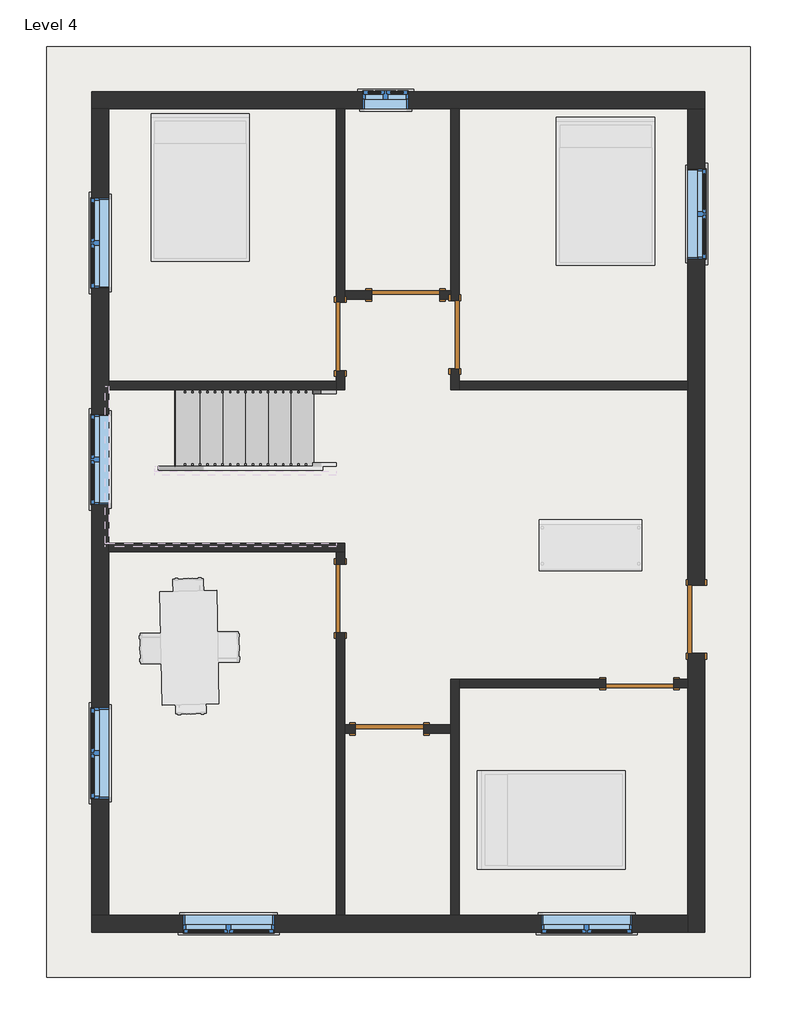
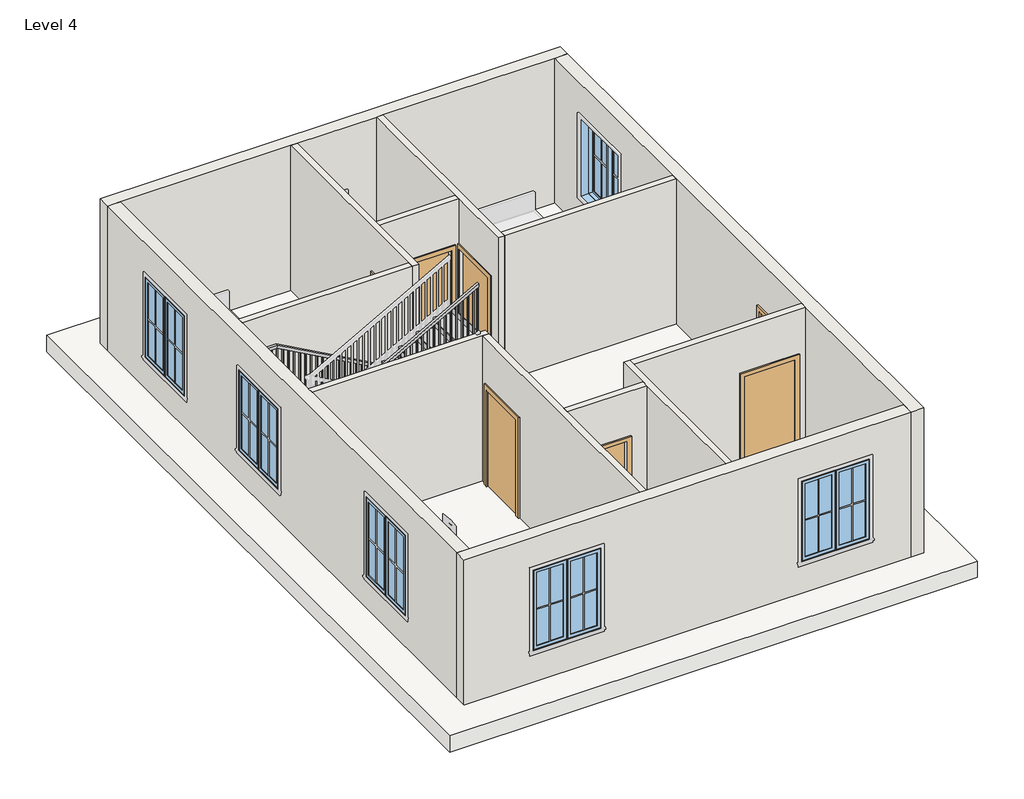
# One storey, part 1 of 2: 14 walls, 7 doors, 7 windows, 1 railing, 1 roof, 1 stair flight.
"""IFC4 building model written with IfcOpenShell, lengths in millimetres."""

from ifc_helpers import new_model, si_unit, frame, origin, place, context, project, spatial, polyline, outline, extrude, faceted_brep, transform, mapped, element, save
from components import door_e5f9f3c4, door_305aa2a5, door_a90ba1ad, stair_flight_3672e095, window_c417fced, window_8377141f

model = new_model("IFC4")

# Units and contexts
model_context = context("Model", 3, world=origin())
ifc_project = project(units=[si_unit("LENGTHUNIT", "METRE", prefix="MILLI")], contexts=[model_context])

# Site, building, storey
site = spatial("IfcSite", under=ifc_project)
building = spatial("IfcBuilding", under=site)
storey = spatial("IfcBuildingStorey", under=building, Name="Level 4", Elevation=9144.0)

# Doors
placement = place(None, origin())
door_shape = door_e5f9f3c4(model_context)
element("IfcDoor", 1, ObjectType="Single-Flush : 36\" x 84\"", at=placement, inside=storey, context=model_context, shape_type="MappedRepresentation", body=[
    mapped(door_shape, transform((5226.05, 11245.85, 9144.0), x_axis=(1.0, 0.0, 0.0), y_axis=(0.0, 1.0, 0.0), z_axis=(0.0, 0.0, 1.0))),
])
element("IfcDoor", 2, ObjectType="Single-Flush : 36\" x 84\"", at=placement, inside=storey, context=model_context, shape_type="MappedRepresentation", body=[
    mapped(door_shape, transform((5886.45, 10712.45, 9144.0), x_axis=(0.0, -1.0, 0.0), y_axis=(1.0, 0.0, 0.0), z_axis=(0.0, 0.0, 1.0))),
])
door_2_shape = door_305aa2a5(model_context)
element("IfcDoor", 3, ObjectType="Single-Flush : 36\" x 84\"", at=placement, inside=storey, context=model_context, shape_type="MappedRepresentation", body=[
    mapped(door_2_shape, transform((4349.75, 10687.05, 9144.0), x_axis=(0.0, -1.0, 0.0), y_axis=(1.0, 0.0, 0.0), z_axis=(0.0, 0.0, 1.0))),
])
element("IfcDoor", 4, ObjectType="Single-Flush : 36\" x 84\"", at=placement, inside=storey, context=model_context, shape_type="MappedRepresentation", body=[
    mapped(door_2_shape, transform((8369.3, 6026.15, 9144.0), x_axis=(1.0, 0.0, 0.0), y_axis=(0.0, 1.0, 0.0), z_axis=(0.0, 0.0, 1.0))),
])
element("IfcDoor", 5, ObjectType="Single-Flush : 36\" x 84\"", at=placement, inside=storey, context=model_context, shape_type="MappedRepresentation", body=[
    mapped(door_2_shape, transform((5010.15, 5416.55, 9144.0), x_axis=(-1.0, 0.0, 0.0), y_axis=(0.0, -1.0, 0.0), z_axis=(0.0, 0.0, 1.0))),
])
element("IfcDoor", 6, ObjectType="Single-Flush : 36\" x 84\"", at=placement, inside=storey, context=model_context, shape_type="MappedRepresentation", body=[
    mapped(door_2_shape, transform((4349.75, 7169.15, 9144.0), x_axis=(0.0, -1.0, 0.0), y_axis=(1.0, 0.0, 0.0), z_axis=(0.0, 0.0, 1.0))),
])
door_3_shape = door_a90ba1ad(model_context)
element("IfcDoor", 7, ObjectType="Single-Flush : 36\" x 84\"", at=placement, inside=storey, context=model_context, shape_type="MappedRepresentation", body=[
    mapped(door_3_shape, transform((9131.3, 6889.75, 9144.0), x_axis=(0.0, -1.0, 0.0), y_axis=(1.0, 0.0, 0.0), z_axis=(0.0, 0.0, 1.0))),
])

# Railing
element("IfcRailing", 8, ObjectType="Handrail - Rectangular", at=placement, inside=storey, context=model_context, shape_type="SolidModel", body=[
    faceted_brep([(4295.1355783, 9918.7, 10227.7333333), (4295.1355783, 9918.7, 10169.620221), (4295.1355783, 9969.5, 10169.620221), (4295.1355783, 9969.5, 10227.7333333), (1856.7355783, 9918.7, 11582.4), (1843.5719761, 9918.7, 11531.6), (1843.5719761, 9969.5, 11531.6), (1856.7355783, 9969.5, 11582.4), (1295.4, 9918.7, 11582.4), (1295.4, 9918.7, 11531.6), (1244.6, 9969.5, 11531.6), (1244.6, 9969.5, 11582.4), (1295.4, 7962.9, 11582.4), (1295.4, 7962.9, 11531.6), (1244.6, 7912.1, 11531.6), (1244.6, 7912.1, 11582.4), (1551.9355783, 7962.9, 11582.4), (1565.0991806, 7962.9, 11531.6), (1565.0991806, 7912.1, 11531.6), (1551.9355783, 7912.1, 11582.4), (4295.1355783, 7962.9, 13106.4), (4295.1355783, 7912.1, 13106.4), (4295.1355783, 7912.1, 13048.2868876), (4295.1355783, 7962.9, 13048.2868876)], [[[0, 1, 2, 3]], [[1, 0, 4, 5]], [[2, 1, 5, 6]], [[3, 2, 6, 7]], [[0, 3, 7, 4]], [[5, 4, 8, 9]], [[6, 5, 9, 10]], [[7, 6, 10, 11]], [[4, 7, 11, 8]], [[9, 8, 12, 13]], [[10, 9, 13, 14]], [[11, 10, 14, 15]], [[8, 11, 15, 12]], [[13, 12, 16, 17]], [[14, 13, 17, 18]], [[15, 14, 18, 19]], [[12, 15, 19, 16]], [[20, 21, 22, 23]], [[17, 16, 20, 23]], [[18, 17, 23, 22]], [[19, 18, 22, 21]], [[16, 19, 21, 20]]]),
    extrude(outline(polyline([(13009.8365664, 4225.925), (12999.253233, 4206.875), (12022.6666667, 4206.875), (12022.6666667, 4225.925), (13009.8365664, 4225.925)])), frame((0.0, 7927.975, 0.0), z_axis=(0.0, 1.0, 0.0), x_axis=(0.0, 0.0, 1.0)), (0.0, 0.0, 1.0), 19.05),
    extrude(outline(polyline([(12953.3921219, 4124.325), (12942.8087886, 4105.275), (12022.6666667, 4105.275), (12022.6666667, 4124.325), (12953.3921219, 4124.325)])), frame((0.0, 7927.975, 0.0), z_axis=(0.0, 1.0, 0.0), x_axis=(0.0, 0.0, 1.0)), (0.0, 0.0, 1.0), 19.05),
    extrude(outline(polyline([(12896.9476775, 4022.725), (12886.3643441, 4003.675), (12022.6666667, 4003.675), (12022.6666667, 4022.725), (12896.9476775, 4022.725)])), frame((0.0, 7927.975, 0.0), z_axis=(0.0, 1.0, 0.0), x_axis=(0.0, 0.0, 1.0)), (0.0, 0.0, 1.0), 19.05),
    extrude(outline(polyline([(12840.503233, 3921.125), (12829.9198997, 3902.075), (11853.3333333, 3902.075), (11853.3333333, 3921.125), (12840.503233, 3921.125)])), frame((0.0, 7927.975, 0.0), z_axis=(0.0, 1.0, 0.0), x_axis=(0.0, 0.0, 1.0)), (0.0, 0.0, 1.0), 19.05),
    extrude(outline(polyline([(12784.0587886, 3819.525), (12773.4754552, 3800.475), (11853.3333333, 3800.475), (11853.3333333, 3819.525), (12784.0587886, 3819.525)])), frame((0.0, 7927.975, 0.0), z_axis=(0.0, 1.0, 0.0), x_axis=(0.0, 0.0, 1.0)), (0.0, 0.0, 1.0), 19.05),
    extrude(outline(polyline([(12727.6143441, 3717.925), (12717.0310108, 3698.875), (11853.3333333, 3698.875), (11853.3333333, 3717.925), (12727.6143441, 3717.925)])), frame((0.0, 7927.975, 0.0), z_axis=(0.0, 1.0, 0.0), x_axis=(0.0, 0.0, 1.0)), (0.0, 0.0, 1.0), 19.05),
    extrude(outline(polyline([(12671.1698997, 3616.325), (12660.5865664, 3597.275), (11684.0, 3597.275), (11684.0, 3616.325), (12671.1698997, 3616.325)])), frame((0.0, 7927.975, 0.0), z_axis=(0.0, 1.0, 0.0), x_axis=(0.0, 0.0, 1.0)), (0.0, 0.0, 1.0), 19.05),
    extrude(outline(polyline([(12614.7254552, 3514.725), (12604.1421219, 3495.675), (11684.0, 3495.675), (11684.0, 3514.725), (12614.7254552, 3514.725)])), frame((0.0, 7927.975, 0.0), z_axis=(0.0, 1.0, 0.0), x_axis=(0.0, 0.0, 1.0)), (0.0, 0.0, 1.0), 19.05),
    extrude(outline(polyline([(12558.2810108, 3413.125), (12547.6976775, 3394.075), (11684.0, 3394.075), (11684.0, 3413.125), (12558.2810108, 3413.125)])), frame((0.0, 7927.975, 0.0), z_axis=(0.0, 1.0, 0.0), x_axis=(0.0, 0.0, 1.0)), (0.0, 0.0, 1.0), 19.05),
    extrude(outline(polyline([(12501.8365664, 3311.525), (12491.253233, 3292.475), (11514.6666667, 3292.475), (11514.6666667, 3311.525), (12501.8365664, 3311.525)])), frame((0.0, 7927.975, 0.0), z_axis=(0.0, 1.0, 0.0), x_axis=(0.0, 0.0, 1.0)), (0.0, 0.0, 1.0), 19.05),
    extrude(outline(polyline([(12445.3921219, 3209.925), (12434.8087886, 3190.875), (11514.6666667, 3190.875), (11514.6666667, 3209.925), (12445.3921219, 3209.925)])), frame((0.0, 7927.975, 0.0), z_axis=(0.0, 1.0, 0.0), x_axis=(0.0, 0.0, 1.0)), (0.0, 0.0, 1.0), 19.05),
    extrude(outline(polyline([(12388.9476775, 3108.325), (12378.3643441, 3089.275), (11514.6666667, 3089.275), (11514.6666667, 3108.325), (12388.9476775, 3108.325)])), frame((0.0, 7927.975, 0.0), z_axis=(0.0, 1.0, 0.0), x_axis=(0.0, 0.0, 1.0)), (0.0, 0.0, 1.0), 19.05),
    extrude(outline(polyline([(12332.503233, 3006.725), (12321.9198997, 2987.675), (11345.3333333, 2987.675), (11345.3333333, 3006.725), (12332.503233, 3006.725)])), frame((0.0, 7927.975, 0.0), z_axis=(0.0, 1.0, 0.0), x_axis=(0.0, 0.0, 1.0)), (0.0, 0.0, 1.0), 19.05),
    extrude(outline(polyline([(12276.0587886, 2905.125), (12265.4754552, 2886.075), (11345.3333333, 2886.075), (11345.3333333, 2905.125), (12276.0587886, 2905.125)])), frame((0.0, 7927.975, 0.0), z_axis=(0.0, 1.0, 0.0), x_axis=(0.0, 0.0, 1.0)), (0.0, 0.0, 1.0), 19.05),
    extrude(outline(polyline([(12219.6143441, 2803.525), (12209.0310108, 2784.475), (11345.3333333, 2784.475), (11345.3333333, 2803.525), (12219.6143441, 2803.525)])), frame((0.0, 7927.975, 0.0), z_axis=(0.0, 1.0, 0.0), x_axis=(0.0, 0.0, 1.0)), (0.0, 0.0, 1.0), 19.05),
    extrude(outline(polyline([(12163.1698997, 2701.925), (12152.5865664, 2682.875), (11176.0, 2682.875), (11176.0, 2701.925), (12163.1698997, 2701.925)])), frame((0.0, 7927.975, 0.0), z_axis=(0.0, 1.0, 0.0), x_axis=(0.0, 0.0, 1.0)), (0.0, 0.0, 1.0), 19.05),
    extrude(outline(polyline([(12106.7254552, 2600.325), (12096.1421219, 2581.275), (11176.0, 2581.275), (11176.0, 2600.325), (12106.7254552, 2600.325)])), frame((0.0, 7927.975, 0.0), z_axis=(0.0, 1.0, 0.0), x_axis=(0.0, 0.0, 1.0)), (0.0, 0.0, 1.0), 19.05),
    extrude(outline(polyline([(12050.2810108, 2498.725), (12039.6976775, 2479.675), (11176.0, 2479.675), (11176.0, 2498.725), (12050.2810108, 2498.725)])), frame((0.0, 7927.975, 0.0), z_axis=(0.0, 1.0, 0.0), x_axis=(0.0, 0.0, 1.0)), (0.0, 0.0, 1.0), 19.05),
    extrude(outline(polyline([(11993.8365664, 2397.125), (11983.253233, 2378.075), (11006.6666667, 2378.075), (11006.6666667, 2397.125), (11993.8365664, 2397.125)])), frame((0.0, 7927.975, 0.0), z_axis=(0.0, 1.0, 0.0), x_axis=(0.0, 0.0, 1.0)), (0.0, 0.0, 1.0), 19.05),
    extrude(outline(polyline([(11937.3921219, 2295.525), (11926.8087886, 2276.475), (11006.6666667, 2276.475), (11006.6666667, 2295.525), (11937.3921219, 2295.525)])), frame((0.0, 7927.975, 0.0), z_axis=(0.0, 1.0, 0.0), x_axis=(0.0, 0.0, 1.0)), (0.0, 0.0, 1.0), 19.05),
    extrude(outline(polyline([(11880.9476775, 2193.925), (11870.3643441, 2174.875), (11006.6666667, 2174.875), (11006.6666667, 2193.925), (11880.9476775, 2193.925)])), frame((0.0, 7927.975, 0.0), z_axis=(0.0, 1.0, 0.0), x_axis=(0.0, 0.0, 1.0)), (0.0, 0.0, 1.0), 19.05),
    extrude(outline(polyline([(11824.503233, 2092.325), (11813.9198997, 2073.275), (10837.3333333, 2073.275), (10837.3333333, 2092.325), (11824.503233, 2092.325)])), frame((0.0, 7927.975, 0.0), z_axis=(0.0, 1.0, 0.0), x_axis=(0.0, 0.0, 1.0)), (0.0, 0.0, 1.0), 19.05),
    extrude(outline(polyline([(11768.0587886, 1990.725), (11757.4754552, 1971.675), (10837.3333333, 1971.675), (10837.3333333, 1990.725), (11768.0587886, 1990.725)])), frame((0.0, 7927.975, 0.0), z_axis=(0.0, 1.0, 0.0), x_axis=(0.0, 0.0, 1.0)), (0.0, 0.0, 1.0), 19.05),
    extrude(outline(polyline([(11711.6143441, 1889.125), (11701.0310108, 1870.075), (10837.3333333, 1870.075), (10837.3333333, 1889.125), (11711.6143441, 1889.125)])), frame((0.0, 7927.975, 0.0), z_axis=(0.0, 1.0, 0.0), x_axis=(0.0, 0.0, 1.0)), (0.0, 0.0, 1.0), 19.05),
    extrude(outline(polyline([(11655.1698997, 1787.525), (11644.5865664, 1768.475), (10668.0, 1768.475), (10668.0, 1787.525), (11655.1698997, 1787.525)])), frame((0.0, 7927.975, 0.0), z_axis=(0.0, 1.0, 0.0), x_axis=(0.0, 0.0, 1.0)), (0.0, 0.0, 1.0), 19.05),
    extrude(outline(polyline([(11598.7254552, 1685.925), (11588.1421219, 1666.875), (10668.0, 1666.875), (10668.0, 1685.925), (11598.7254552, 1685.925)])), frame((0.0, 7927.975, 0.0), z_axis=(0.0, 1.0, 0.0), x_axis=(0.0, 0.0, 1.0)), (0.0, 0.0, 1.0), 19.05),
    extrude(outline(polyline([(11542.2810108, 1584.325), (11531.6976775, 1565.275), (10668.0, 1565.275), (10668.0, 1584.325), (11542.2810108, 1584.325)])), frame((0.0, 7927.975, 0.0), z_axis=(0.0, 1.0, 0.0), x_axis=(0.0, 0.0, 1.0)), (0.0, 0.0, 1.0), 19.05),
    extrude(outline(polyline([(1463.675, 7927.975), (1463.675, 7947.025), (1482.725, 7947.025), (1482.725, 7927.975), (1463.675, 7927.975)])), frame((0.0, 0.0, 10668.0), z_axis=(0.0, 0.0, 1.0), x_axis=(1.0, 0.0, 0.0)), (0.0, 0.0, 1.0), 863.6),
    extrude(outline(polyline([(1362.075, 7927.975), (1362.075, 7947.025), (1381.125, 7947.025), (1381.125, 7927.975), (1362.075, 7927.975)])), frame((0.0, 0.0, 10668.0), z_axis=(0.0, 0.0, 1.0), x_axis=(1.0, 0.0, 0.0)), (0.0, 0.0, 1.0), 863.6),
    extrude(outline(polyline([(1260.475, 8023.225), (1279.525, 8023.225), (1279.525, 8004.175), (1260.475, 8004.175), (1260.475, 8023.225)])), frame((0.0, 0.0, 10668.0), z_axis=(0.0, 0.0, 1.0), x_axis=(1.0, 0.0, 0.0)), (0.0, 0.0, 1.0), 863.6),
    extrude(outline(polyline([(1260.475, 8124.825), (1279.525, 8124.825), (1279.525, 8105.775), (1260.475, 8105.775), (1260.475, 8124.825)])), frame((0.0, 0.0, 10668.0), z_axis=(0.0, 0.0, 1.0), x_axis=(1.0, 0.0, 0.0)), (0.0, 0.0, 1.0), 863.6),
    extrude(outline(polyline([(1260.475, 8226.425), (1279.525, 8226.425), (1279.525, 8207.375), (1260.475, 8207.375), (1260.475, 8226.425)])), frame((0.0, 0.0, 10668.0), z_axis=(0.0, 0.0, 1.0), x_axis=(1.0, 0.0, 0.0)), (0.0, 0.0, 1.0), 863.6),
    extrude(outline(polyline([(1260.475, 8328.025), (1279.525, 8328.025), (1279.525, 8308.975), (1260.475, 8308.975), (1260.475, 8328.025)])), frame((0.0, 0.0, 10668.0), z_axis=(0.0, 0.0, 1.0), x_axis=(1.0, 0.0, 0.0)), (0.0, 0.0, 1.0), 863.6),
    extrude(outline(polyline([(1260.475, 8429.625), (1279.525, 8429.625), (1279.525, 8410.575), (1260.475, 8410.575), (1260.475, 8429.625)])), frame((0.0, 0.0, 10668.0), z_axis=(0.0, 0.0, 1.0), x_axis=(1.0, 0.0, 0.0)), (0.0, 0.0, 1.0), 863.6),
    extrude(outline(polyline([(1260.475, 8531.225), (1279.525, 8531.225), (1279.525, 8512.175), (1260.475, 8512.175), (1260.475, 8531.225)])), frame((0.0, 0.0, 10668.0), z_axis=(0.0, 0.0, 1.0), x_axis=(1.0, 0.0, 0.0)), (0.0, 0.0, 1.0), 863.6),
    extrude(outline(polyline([(1260.475, 8632.825), (1279.525, 8632.825), (1279.525, 8613.775), (1260.475, 8613.775), (1260.475, 8632.825)])), frame((0.0, 0.0, 10668.0), z_axis=(0.0, 0.0, 1.0), x_axis=(1.0, 0.0, 0.0)), (0.0, 0.0, 1.0), 863.6),
    extrude(outline(polyline([(1260.475, 8734.425), (1279.525, 8734.425), (1279.525, 8715.375), (1260.475, 8715.375), (1260.475, 8734.425)])), frame((0.0, 0.0, 10668.0), z_axis=(0.0, 0.0, 1.0), x_axis=(1.0, 0.0, 0.0)), (0.0, 0.0, 1.0), 863.6),
    extrude(outline(polyline([(1260.475, 8836.025), (1279.525, 8836.025), (1279.525, 8816.975), (1260.475, 8816.975), (1260.475, 8836.025)])), frame((0.0, 0.0, 10668.0), z_axis=(0.0, 0.0, 1.0), x_axis=(1.0, 0.0, 0.0)), (0.0, 0.0, 1.0), 863.6),
    extrude(outline(polyline([(1260.475, 8937.625), (1279.525, 8937.625), (1279.525, 8918.575), (1260.475, 8918.575), (1260.475, 8937.625)])), frame((0.0, 0.0, 10668.0), z_axis=(0.0, 0.0, 1.0), x_axis=(1.0, 0.0, 0.0)), (0.0, 0.0, 1.0), 863.6),
    extrude(outline(polyline([(1260.475, 9039.225), (1279.525, 9039.225), (1279.525, 9020.175), (1260.475, 9020.175), (1260.475, 9039.225)])), frame((0.0, 0.0, 10668.0), z_axis=(0.0, 0.0, 1.0), x_axis=(1.0, 0.0, 0.0)), (0.0, 0.0, 1.0), 863.6),
    extrude(outline(polyline([(1260.475, 9140.825), (1279.525, 9140.825), (1279.525, 9121.775), (1260.475, 9121.775), (1260.475, 9140.825)])), frame((0.0, 0.0, 10668.0), z_axis=(0.0, 0.0, 1.0), x_axis=(1.0, 0.0, 0.0)), (0.0, 0.0, 1.0), 863.6),
    extrude(outline(polyline([(1260.475, 9242.425), (1279.525, 9242.425), (1279.525, 9223.375), (1260.475, 9223.375), (1260.475, 9242.425)])), frame((0.0, 0.0, 10668.0), z_axis=(0.0, 0.0, 1.0), x_axis=(1.0, 0.0, 0.0)), (0.0, 0.0, 1.0), 863.6),
    extrude(outline(polyline([(1260.475, 9344.025), (1279.525, 9344.025), (1279.525, 9324.975), (1260.475, 9324.975), (1260.475, 9344.025)])), frame((0.0, 0.0, 10668.0), z_axis=(0.0, 0.0, 1.0), x_axis=(1.0, 0.0, 0.0)), (0.0, 0.0, 1.0), 863.6),
    extrude(outline(polyline([(1260.475, 9445.625), (1279.525, 9445.625), (1279.525, 9426.575), (1260.475, 9426.575), (1260.475, 9445.625)])), frame((0.0, 0.0, 10668.0), z_axis=(0.0, 0.0, 1.0), x_axis=(1.0, 0.0, 0.0)), (0.0, 0.0, 1.0), 863.6),
    extrude(outline(polyline([(1260.475, 9547.225), (1279.525, 9547.225), (1279.525, 9528.175), (1260.475, 9528.175), (1260.475, 9547.225)])), frame((0.0, 0.0, 10668.0), z_axis=(0.0, 0.0, 1.0), x_axis=(1.0, 0.0, 0.0)), (0.0, 0.0, 1.0), 863.6),
    extrude(outline(polyline([(1260.475, 9648.825), (1279.525, 9648.825), (1279.525, 9629.775), (1260.475, 9629.775), (1260.475, 9648.825)])), frame((0.0, 0.0, 10668.0), z_axis=(0.0, 0.0, 1.0), x_axis=(1.0, 0.0, 0.0)), (0.0, 0.0, 1.0), 863.6),
    extrude(outline(polyline([(1260.475, 9750.425), (1279.525, 9750.425), (1279.525, 9731.375), (1260.475, 9731.375), (1260.475, 9750.425)])), frame((0.0, 0.0, 10668.0), z_axis=(0.0, 0.0, 1.0), x_axis=(1.0, 0.0, 0.0)), (0.0, 0.0, 1.0), 863.6),
    extrude(outline(polyline([(1260.475, 9852.025), (1279.525, 9852.025), (1279.525, 9832.975), (1260.475, 9832.975), (1260.475, 9852.025)])), frame((0.0, 0.0, 10668.0), z_axis=(0.0, 0.0, 1.0), x_axis=(1.0, 0.0, 0.0)), (0.0, 0.0, 1.0), 863.6),
    extrude(outline(polyline([(1358.2605783, 9953.625), (1358.2605783, 9934.575), (1339.2105783, 9934.575), (1339.2105783, 9953.625), (1358.2605783, 9953.625)])), frame((0.0, 0.0, 10668.0), z_axis=(0.0, 0.0, 1.0), x_axis=(1.0, 0.0, 0.0)), (0.0, 0.0, 1.0), 863.6),
    extrude(outline(polyline([(1459.8605783, 9953.625), (1459.8605783, 9934.575), (1440.8105783, 9934.575), (1440.8105783, 9953.625), (1459.8605783, 9953.625)])), frame((0.0, 0.0, 10668.0), z_axis=(0.0, 0.0, 1.0), x_axis=(1.0, 0.0, 0.0)), (0.0, 0.0, 1.0), 863.6),
    extrude(outline(polyline([(1561.4605783, 9953.625), (1561.4605783, 9934.575), (1542.4105783, 9934.575), (1542.4105783, 9953.625), (1561.4605783, 9953.625)])), frame((0.0, 0.0, 10668.0), z_axis=(0.0, 0.0, 1.0), x_axis=(1.0, 0.0, 0.0)), (0.0, 0.0, 1.0), 863.6),
    extrude(outline(polyline([(1663.0605783, 9953.625), (1663.0605783, 9934.575), (1644.0105783, 9934.575), (1644.0105783, 9953.625), (1663.0605783, 9953.625)])), frame((0.0, 0.0, 10668.0), z_axis=(0.0, 0.0, 1.0), x_axis=(1.0, 0.0, 0.0)), (0.0, 0.0, 1.0), 863.6),
    extrude(outline(polyline([(1764.6605783, 9953.625), (1764.6605783, 9934.575), (1745.6105783, 9934.575), (1745.6105783, 9953.625), (1764.6605783, 9953.625)])), frame((0.0, 0.0, 10668.0), z_axis=(0.0, 0.0, 1.0), x_axis=(1.0, 0.0, 0.0)), (0.0, 0.0, 1.0), 863.6),
    extrude(outline(polyline([(11518.995221, 1866.2605783), (11529.5785543, 1847.2105783), (10668.0, 1847.2105783), (10668.0, 1866.2605783), (11518.995221, 1866.2605783)])), frame((0.0, 9934.575, 0.0), z_axis=(0.0, 1.0, 0.0), x_axis=(0.0, 0.0, 1.0)), (0.0, 0.0, 1.0), 19.05),
    extrude(outline(polyline([(11462.5507765, 1967.8605783), (11473.1341099, 1948.8105783), (10498.6666667, 1948.8105783), (10498.6666667, 1967.8605783), (11462.5507765, 1967.8605783)])), frame((0.0, 9934.575, 0.0), z_axis=(0.0, 1.0, 0.0), x_axis=(0.0, 0.0, 1.0)), (0.0, 0.0, 1.0), 19.05),
    extrude(outline(polyline([(11406.1063321, 2069.4605783), (11416.6896654, 2050.4105783), (10498.6666667, 2050.4105783), (10498.6666667, 2069.4605783), (11406.1063321, 2069.4605783)])), frame((0.0, 9934.575, 0.0), z_axis=(0.0, 1.0, 0.0), x_axis=(0.0, 0.0, 1.0)), (0.0, 0.0, 1.0), 19.05),
    extrude(outline(polyline([(11349.6618876, 2171.0605783), (11360.245221, 2152.0105783), (10498.6666667, 2152.0105783), (10498.6666667, 2171.0605783), (11349.6618876, 2171.0605783)])), frame((0.0, 9934.575, 0.0), z_axis=(0.0, 1.0, 0.0), x_axis=(0.0, 0.0, 1.0)), (0.0, 0.0, 1.0), 19.05),
    extrude(outline(polyline([(11293.2174432, 2272.6605783), (11303.8007765, 2253.6105783), (10329.3333333, 2253.6105783), (10329.3333333, 2272.6605783), (11293.2174432, 2272.6605783)])), frame((0.0, 9934.575, 0.0), z_axis=(0.0, 1.0, 0.0), x_axis=(0.0, 0.0, 1.0)), (0.0, 0.0, 1.0), 19.05),
    extrude(outline(polyline([(11236.7729988, 2374.2605783), (11247.3563321, 2355.2105783), (10329.3333333, 2355.2105783), (10329.3333333, 2374.2605783), (11236.7729988, 2374.2605783)])), frame((0.0, 9934.575, 0.0), z_axis=(0.0, 1.0, 0.0), x_axis=(0.0, 0.0, 1.0)), (0.0, 0.0, 1.0), 19.05),
    extrude(outline(polyline([(11180.3285543, 2475.8605783), (11190.9118876, 2456.8105783), (10329.3333333, 2456.8105783), (10329.3333333, 2475.8605783), (11180.3285543, 2475.8605783)])), frame((0.0, 9934.575, 0.0), z_axis=(0.0, 1.0, 0.0), x_axis=(0.0, 0.0, 1.0)), (0.0, 0.0, 1.0), 19.05),
    extrude(outline(polyline([(11123.8841099, 2577.4605783), (11134.4674432, 2558.4105783), (10160.0, 2558.4105783), (10160.0, 2577.4605783), (11123.8841099, 2577.4605783)])), frame((0.0, 9934.575, 0.0), z_axis=(0.0, 1.0, 0.0), x_axis=(0.0, 0.0, 1.0)), (0.0, 0.0, 1.0), 19.05),
    extrude(outline(polyline([(11067.4396654, 2679.0605783), (11078.0229988, 2660.0105783), (10160.0, 2660.0105783), (10160.0, 2679.0605783), (11067.4396654, 2679.0605783)])), frame((0.0, 9934.575, 0.0), z_axis=(0.0, 1.0, 0.0), x_axis=(0.0, 0.0, 1.0)), (0.0, 0.0, 1.0), 19.05),
    extrude(outline(polyline([(11010.995221, 2780.6605783), (11021.5785543, 2761.6105783), (10160.0, 2761.6105783), (10160.0, 2780.6605783), (11010.995221, 2780.6605783)])), frame((0.0, 9934.575, 0.0), z_axis=(0.0, 1.0, 0.0), x_axis=(0.0, 0.0, 1.0)), (0.0, 0.0, 1.0), 19.05),
    extrude(outline(polyline([(10954.5507765, 2882.2605783), (10965.1341099, 2863.2105783), (9990.6666667, 2863.2105783), (9990.6666667, 2882.2605783), (10954.5507765, 2882.2605783)])), frame((0.0, 9934.575, 0.0), z_axis=(0.0, 1.0, 0.0), x_axis=(0.0, 0.0, 1.0)), (0.0, 0.0, 1.0), 19.05),
    extrude(outline(polyline([(10898.1063321, 2983.8605783), (10908.6896654, 2964.8105783), (9990.6666667, 2964.8105783), (9990.6666667, 2983.8605783), (10898.1063321, 2983.8605783)])), frame((0.0, 9934.575, 0.0), z_axis=(0.0, 1.0, 0.0), x_axis=(0.0, 0.0, 1.0)), (0.0, 0.0, 1.0), 19.05),
    extrude(outline(polyline([(10841.6618876, 3085.4605783), (10852.245221, 3066.4105783), (9990.6666667, 3066.4105783), (9990.6666667, 3085.4605783), (10841.6618876, 3085.4605783)])), frame((0.0, 9934.575, 0.0), z_axis=(0.0, 1.0, 0.0), x_axis=(0.0, 0.0, 1.0)), (0.0, 0.0, 1.0), 19.05),
    extrude(outline(polyline([(10785.2174432, 3187.0605783), (10795.8007765, 3168.0105783), (9821.3333333, 3168.0105783), (9821.3333333, 3187.0605783), (10785.2174432, 3187.0605783)])), frame((0.0, 9934.575, 0.0), z_axis=(0.0, 1.0, 0.0), x_axis=(0.0, 0.0, 1.0)), (0.0, 0.0, 1.0), 19.05),
    extrude(outline(polyline([(10728.7729988, 3288.6605783), (10739.3563321, 3269.6105783), (9821.3333333, 3269.6105783), (9821.3333333, 3288.6605783), (10728.7729988, 3288.6605783)])), frame((0.0, 9934.575, 0.0), z_axis=(0.0, 1.0, 0.0), x_axis=(0.0, 0.0, 1.0)), (0.0, 0.0, 1.0), 19.05),
    extrude(outline(polyline([(10672.3285543, 3390.2605783), (10682.9118876, 3371.2105783), (9821.3333333, 3371.2105783), (9821.3333333, 3390.2605783), (10672.3285543, 3390.2605783)])), frame((0.0, 9934.575, 0.0), z_axis=(0.0, 1.0, 0.0), x_axis=(0.0, 0.0, 1.0)), (0.0, 0.0, 1.0), 19.05),
    extrude(outline(polyline([(10615.8841099, 3491.8605783), (10626.4674432, 3472.8105783), (9652.0, 3472.8105783), (9652.0, 3491.8605783), (10615.8841099, 3491.8605783)])), frame((0.0, 9934.575, 0.0), z_axis=(0.0, 1.0, 0.0), x_axis=(0.0, 0.0, 1.0)), (0.0, 0.0, 1.0), 19.05),
    extrude(outline(polyline([(10559.4396654, 3593.4605783), (10570.0229988, 3574.4105783), (9652.0, 3574.4105783), (9652.0, 3593.4605783), (10559.4396654, 3593.4605783)])), frame((0.0, 9934.575, 0.0), z_axis=(0.0, 1.0, 0.0), x_axis=(0.0, 0.0, 1.0)), (0.0, 0.0, 1.0), 19.05),
    extrude(outline(polyline([(10502.995221, 3695.0605783), (10513.5785543, 3676.0105783), (9652.0, 3676.0105783), (9652.0, 3695.0605783), (10502.995221, 3695.0605783)])), frame((0.0, 9934.575, 0.0), z_axis=(0.0, 1.0, 0.0), x_axis=(0.0, 0.0, 1.0)), (0.0, 0.0, 1.0), 19.05),
    extrude(outline(polyline([(10446.5507765, 3796.6605783), (10457.1341099, 3777.6105783), (9482.6666667, 3777.6105783), (9482.6666667, 3796.6605783), (10446.5507765, 3796.6605783)])), frame((0.0, 9934.575, 0.0), z_axis=(0.0, 1.0, 0.0), x_axis=(0.0, 0.0, 1.0)), (0.0, 0.0, 1.0), 19.05),
    extrude(outline(polyline([(10390.1063321, 3898.2605783), (10400.6896654, 3879.2105783), (9482.6666667, 3879.2105783), (9482.6666667, 3898.2605783), (10390.1063321, 3898.2605783)])), frame((0.0, 9934.575, 0.0), z_axis=(0.0, 1.0, 0.0), x_axis=(0.0, 0.0, 1.0)), (0.0, 0.0, 1.0), 19.05),
    extrude(outline(polyline([(10333.6618876, 3999.8605783), (10344.245221, 3980.8105783), (9482.6666667, 3980.8105783), (9482.6666667, 3999.8605783), (10333.6618876, 3999.8605783)])), frame((0.0, 9934.575, 0.0), z_axis=(0.0, 1.0, 0.0), x_axis=(0.0, 0.0, 1.0)), (0.0, 0.0, 1.0), 19.05),
    extrude(outline(polyline([(10277.2174432, 4101.4605783), (10287.8007765, 4082.4105783), (9313.3333333, 4082.4105783), (9313.3333333, 4101.4605783), (10277.2174432, 4101.4605783)])), frame((0.0, 9934.575, 0.0), z_axis=(0.0, 1.0, 0.0), x_axis=(0.0, 0.0, 1.0)), (0.0, 0.0, 1.0), 19.05),
    extrude(outline(polyline([(10220.7729988, 4203.0605783), (10231.3563321, 4184.0105783), (9313.3333333, 4184.0105783), (9313.3333333, 4203.0605783), (10220.7729988, 4203.0605783)])), frame((0.0, 9934.575, 0.0), z_axis=(0.0, 1.0, 0.0), x_axis=(0.0, 0.0, 1.0)), (0.0, 0.0, 1.0), 19.05),
    extrude(outline(polyline([(1260.475, 7947.025), (1279.525, 7947.025), (1279.525, 7927.975), (1260.475, 7927.975), (1260.475, 7947.025)])), frame((0.0, 0.0, 10668.0), z_axis=(0.0, 0.0, 1.0), x_axis=(1.0, 0.0, 0.0)), (0.0, 0.0, 1.0), 863.6),
    extrude(outline(polyline([(1279.525, 9953.625), (1279.525, 9934.575), (1260.475, 9934.575), (1260.475, 9953.625), (1279.525, 9953.625)])), frame((0.0, 0.0, 10668.0), z_axis=(0.0, 0.0, 1.0), x_axis=(1.0, 0.0, 0.0)), (0.0, 0.0, 1.0), 863.6),
    extrude(outline(polyline([(13048.2868876, 4295.1355783), (13037.7035543, 4276.0855783), (12022.6666667, 4276.0855783), (12022.6666667, 4295.1355783), (13048.2868876, 4295.1355783)])), frame((0.0, 7927.975, 0.0), z_axis=(0.0, 1.0, 0.0), x_axis=(0.0, 0.0, 1.0)), (0.0, 0.0, 1.0), 19.05),
    extrude(outline(polyline([(10169.620221, 4295.1355783), (10180.2035543, 4276.0855783), (9313.3333333, 4276.0855783), (9313.3333333, 4295.1355783), (10169.620221, 4295.1355783)])), frame((0.0, 9934.575, 0.0), z_axis=(0.0, 1.0, 0.0), x_axis=(0.0, 0.0, 1.0)), (0.0, 0.0, 1.0), 19.05),
])

# Roof
element("IfcRoof", 9, ObjectType="Generic - 12\"", at=placement, inside=storey, context=model_context, shape_type="SweptSolid", body=[
    extrude(outline(polyline([(406.4, 14579.6), (9855.2, 14579.6), (9855.2, 2082.8), (406.4, 2082.8), (406.4, 14579.6)])), frame((0.0, 0.0, 9144.0), z_axis=(0.0, 0.0, 1.0), x_axis=(1.0, 0.0, 0.0)), (0.0, 0.0, 1.0), 304.8),
])

# Stair flight
stair_flight_shape = stair_flight_3672e095(model_context)
element("IfcStairFlight", 10, ObjectType="2\" Tread 1\" Nosing 1/4\" Riser", at=placement, inside=storey, context=model_context, shape_type="MappedRepresentation", body=[
    mapped(stair_flight_shape, transform((0.0, 0.0, 0.0), x_axis=(1.0, 0.0, 0.0), y_axis=(0.0, 1.0, 0.0), z_axis=(0.0, 0.0, 1.0))),
])

# Walls
element("IfcWall", 11, ObjectType="Generic - 5\"", at=placement, inside=storey, context=model_context, shape_type="Brep", body=[
    faceted_brep([(4292.6, 10229.85, 11277.6), (4292.6, 10229.85, 9144.0), (4292.6, 10083.8, 9144.0), (4292.6, 9969.5, 9144.0), (4292.6, 9969.5, 12192.0), (4292.6, 10083.8, 12192.0), (4292.6, 13741.4, 12192.0), (4292.6, 13741.4, 9144.0), (4292.6, 11144.25, 9144.0), (4292.6, 11144.25, 11277.6), (4406.9, 9969.5, 9144.0), (4406.9, 10229.85, 9144.0), (4406.9, 10229.85, 11277.6), (4406.9, 11144.25, 11277.6), (4406.9, 11144.25, 9144.0), (4406.9, 11188.7, 9144.0), (4406.9, 11303.0, 9144.0), (4406.9, 13741.4, 9144.0), (4406.9, 13741.4, 12192.0), (4406.9, 11303.0, 12192.0), (4406.9, 11188.7, 12192.0), (4406.9, 9969.5, 12192.0)], [[[0, 1, 2, 3, 4, 5, 6, 7, 8, 9]], [[10, 11, 12, 13, 14, 15, 16, 17, 18, 19, 20, 21]], [[8, 7, 17, 16, 15, 14]], [[3, 2, 1, 11, 10]], [[6, 5, 4, 21, 20, 19, 18]], [[7, 6, 18, 17]], [[4, 3, 10, 21]], [[12, 11, 1, 0]], [[13, 12, 0, 9]], [[14, 13, 9, 8]]]),
])
element("IfcWall", 12, ObjectType="Generic - 5\"", at=placement, inside=storey, context=model_context, shape_type="SweptSolid", body=[
    extrude(outline(polyline([(1244.6, 10083.8), (4292.6, 10083.8), (4292.6, 9969.5), (1244.6, 9969.5), (1244.6, 10083.8)])), frame((0.0, 0.0, 9144.0), z_axis=(0.0, 0.0, 1.0), x_axis=(1.0, 0.0, 0.0)), (0.0, 0.0, 1.0), 3048.0),
])
element("IfcWall", 13, ObjectType="Generic - 5\"", at=placement, inside=storey, context=model_context, shape_type="SweptSolid", body=[
    extrude(outline(polyline([(11277.6, 5683.25), (9144.0, 5683.25), (9144.0, 5829.3), (12192.0, 5829.3), (12192.0, 4406.9), (9144.0, 4406.9), (9144.0, 4768.85), (11277.6, 4768.85), (11277.6, 5683.25)])), frame((0.0, 11188.7, 0.0), z_axis=(0.0, 1.0, 0.0), x_axis=(0.0, 0.0, 1.0)), (0.0, 0.0, 1.0), 114.3),
])
element("IfcWall", 14, ObjectType="Generic - 5\"", at=placement, inside=storey, context=model_context, shape_type="Brep", body=[
    faceted_brep([(5829.3, 10255.25, 11277.6), (5829.3, 10255.25, 9144.0), (5829.3, 9969.5, 9144.0), (5829.3, 9969.5, 12192.0), (5829.3, 11188.7, 12192.0), (5829.3, 11303.0, 12192.0), (5829.3, 13741.4, 12192.0), (5829.3, 13741.4, 9144.0), (5829.3, 11303.0, 9144.0), (5829.3, 11188.7, 9144.0), (5829.3, 11169.65, 9144.0), (5829.3, 11169.65, 11277.6), (5943.6, 9969.5, 9144.0), (5943.6, 10083.8, 9144.0), (5943.6, 10255.25, 9144.0), (5943.6, 10255.25, 11277.6), (5943.6, 11169.65, 11277.6), (5943.6, 11169.65, 9144.0), (5943.6, 13741.4, 9144.0), (5943.6, 13741.4, 12192.0), (5943.6, 10083.8, 12192.0), (5943.6, 9969.5, 12192.0)], [[[0, 1, 2, 3, 4, 5, 6, 7, 8, 9, 10, 11]], [[12, 13, 14, 15, 16, 17, 18, 19, 20, 21]], [[2, 1, 14, 13, 12]], [[10, 9, 8, 7, 18, 17]], [[6, 5, 4, 3, 21, 20, 19]], [[7, 6, 19, 18]], [[3, 2, 12, 21]], [[15, 14, 1, 0]], [[16, 15, 0, 11]], [[17, 16, 11, 10]]]),
])
element("IfcWall", 15, ObjectType="Generic - 5\"", at=placement, inside=storey, context=model_context, shape_type="SweptSolid", body=[
    extrude(outline(polyline([(9017.0, 9969.5), (5943.6, 9969.5), (5943.6, 10083.8), (9017.0, 10083.8), (9017.0, 9969.5)])), frame((0.0, 0.0, 9144.0), z_axis=(0.0, 0.0, 1.0), x_axis=(1.0, 0.0, 0.0)), (0.0, 0.0, 1.0), 3048.0),
])
element("IfcWall", 16, ObjectType="Generic - 5\"", at=placement, inside=storey, context=model_context, shape_type="Brep", body=[
    faceted_brep([(1244.6, 7797.8, 9144.0), (4292.6, 7797.8, 9144.0), (4406.9, 7797.8, 9144.0), (4406.9, 7797.8, 12192.0), (4292.6, 7797.8, 12192.0), (1244.6, 7797.8, 12192.0), (1244.6, 7912.1, 9144.0), (1244.6, 7912.1, 12192.0), (4406.9, 7912.1, 12192.0), (4406.9, 7912.1, 9144.0)], [[[0, 1, 2, 3, 4, 5]], [[6, 7, 8, 9]], [[2, 1, 0, 6, 9]], [[5, 4, 3, 8, 7]], [[0, 5, 7, 6]], [[3, 2, 9, 8]]]),
])
element("IfcWall", 17, ObjectType="Generic - 5\"", at=placement, inside=storey, context=model_context, shape_type="Brep", body=[
    faceted_brep([(4292.6, 6711.95, 11277.6), (4292.6, 6711.95, 9144.0), (4292.6, 2921.0, 9144.0), (4292.6, 2921.0, 12192.0), (4292.6, 7797.8, 12192.0), (4292.6, 7797.8, 9144.0), (4292.6, 7626.35, 9144.0), (4292.6, 7626.35, 11277.6), (4406.9, 2921.0, 9144.0), (4406.9, 5359.4, 9144.0), (4406.9, 5473.7, 9144.0), (4406.9, 6711.95, 9144.0), (4406.9, 6711.95, 11277.6), (4406.9, 7626.35, 11277.6), (4406.9, 7626.35, 9144.0), (4406.9, 7797.8, 9144.0), (4406.9, 7797.8, 12192.0), (4406.9, 5473.7, 12192.0), (4406.9, 5359.4, 12192.0), (4406.9, 2921.0, 12192.0)], [[[0, 1, 2, 3, 4, 5, 6, 7]], [[8, 9, 10, 11, 12, 13, 14, 15, 16, 17, 18, 19]], [[6, 5, 15, 14]], [[2, 1, 11, 10, 9, 8]], [[4, 3, 19, 18, 17, 16]], [[5, 4, 16, 15]], [[3, 2, 8, 19]], [[12, 11, 1, 0]], [[13, 12, 0, 7]], [[14, 13, 7, 6]]]),
])
element("IfcWall", 18, ObjectType="Generic - 5\"", at=placement, inside=storey, context=model_context, shape_type="SweptSolid", body=[
    extrude(outline(polyline([(9144.0, 4406.9), (9144.0, 4552.95), (11277.6, 4552.95), (11277.6, 5467.35), (9144.0, 5467.35), (9144.0, 5829.3), (12192.0, 5829.3), (12192.0, 4406.9), (9144.0, 4406.9)])), frame((0.0, 5359.4, 0.0), z_axis=(0.0, 1.0, 0.0), x_axis=(0.0, 0.0, 1.0)), (0.0, 0.0, 1.0), 114.3),
])
element("IfcWall", 19, ObjectType="Generic - 5\"", at=placement, inside=storey, context=model_context, shape_type="Brep", body=[
    faceted_brep([(5943.6, 2921.0, 9144.0), (5943.6, 5969.0, 9144.0), (5943.6, 6083.3, 9144.0), (5943.6, 6083.3, 12192.0), (5943.6, 5969.0, 12192.0), (5943.6, 2921.0, 12192.0), (5829.3, 2921.0, 9144.0), (5829.3, 2921.0, 12192.0), (5829.3, 5359.4, 12192.0), (5829.3, 5473.7, 12192.0), (5829.3, 6083.3, 12192.0), (5829.3, 6083.3, 9144.0), (5829.3, 5473.7, 9144.0), (5829.3, 5359.4, 9144.0)], [[[0, 1, 2, 3, 4, 5]], [[6, 7, 8, 9, 10, 11, 12, 13]], [[2, 1, 0, 6, 13, 12, 11]], [[5, 4, 3, 10, 9, 8, 7]], [[0, 5, 7, 6]], [[3, 2, 11, 10]]]),
])
element("IfcWall", 20, ObjectType="Generic - 5\"", at=placement, inside=storey, context=model_context, shape_type="SweptSolid", body=[
    extrude(outline(polyline([(11277.6, 8826.5), (9144.0, 8826.5), (9144.0, 9017.0), (12192.0, 9017.0), (12192.0, 5943.6), (9144.0, 5943.6), (9144.0, 7912.1), (11277.6, 7912.1), (11277.6, 8826.5)])), frame((0.0, 5969.0, 0.0), z_axis=(0.0, 1.0, 0.0), x_axis=(0.0, 0.0, 1.0)), (0.0, 0.0, 1.0), 114.3),
])
element("IfcWall", 21, ObjectType="Generic - 8\"", at=placement, inside=storey, context=model_context, shape_type="Brep", body=[
    faceted_brep([(1016.0, 13741.4, 9144.0), (1244.6, 13741.4, 9144.0), (4292.6, 13741.4, 9144.0), (4406.9, 13741.4, 9144.0), (5829.3, 13741.4, 9144.0), (5943.6, 13741.4, 9144.0), (9017.0, 13741.4, 9144.0), (9245.6, 13741.4, 9144.0), (9245.6, 13741.4, 12192.0), (9017.0, 13741.4, 12192.0), (5943.6, 13741.4, 12192.0), (5829.3, 13741.4, 12192.0), (4406.9, 13741.4, 12192.0), (4292.6, 13741.4, 12192.0), (1244.6, 13741.4, 12192.0), (1016.0, 13741.4, 12192.0), (5264.15, 13741.4, 10972.8), (5264.15, 13741.4, 10058.4), (4654.55, 13741.4, 10058.4), (4654.55, 13741.4, 10972.8), (1016.0, 13970.0, 9144.0), (1016.0, 13970.0, 12192.0), (9245.6, 13970.0, 12192.0), (9245.6, 13970.0, 9144.0), (5264.15, 13970.0, 10972.8), (4654.55, 13970.0, 10972.8), (4654.55, 13970.0, 10058.4), (5264.15, 13970.0, 10058.4)], [[[0, 1, 2, 3, 4, 5, 6, 7, 8, 9, 10, 11, 12, 13, 14, 15], [16, 17, 18, 19]], [[20, 21, 22, 23], [24, 25, 26, 27]], [[7, 6, 5, 4, 3, 2, 1, 0, 20, 23]], [[15, 14, 13, 12, 11, 10, 9, 8, 22, 21]], [[8, 7, 23, 22]], [[0, 15, 21, 20]], [[17, 16, 24, 27]], [[18, 17, 27, 26]], [[19, 18, 26, 25]], [[16, 19, 25, 24]]]),
])
element("IfcWall", 22, ObjectType="Generic - 8\"", at=placement, inside=storey, context=model_context, shape_type="Brep", body=[
    faceted_brep([(9017.0, 6432.55, 11277.6), (9017.0, 6432.55, 9144.0), (9017.0, 6083.3, 9144.0), (9017.0, 5969.0, 9144.0), (9017.0, 2921.0, 9144.0), (9017.0, 2692.4, 9144.0), (9017.0, 2692.4, 12192.0), (9017.0, 2921.0, 12192.0), (9017.0, 5969.0, 12192.0), (9017.0, 6083.3, 12192.0), (9017.0, 9969.5, 12192.0), (9017.0, 10083.8, 12192.0), (9017.0, 13741.4, 12192.0), (9017.0, 13741.4, 9144.0), (9017.0, 10083.8, 9144.0), (9017.0, 9969.5, 9144.0), (9017.0, 7346.95, 9144.0), (9017.0, 7346.95, 11277.6), (9017.0, 11722.1, 11582.4), (9017.0, 11722.1, 10058.4), (9017.0, 12941.3, 10058.4), (9017.0, 12941.3, 11582.4), (9245.6, 2692.4, 9144.0), (9245.6, 6432.55, 9144.0), (9245.6, 6432.55, 11277.6), (9245.6, 7346.95, 11277.6), (9245.6, 7346.95, 9144.0), (9245.6, 13741.4, 9144.0), (9245.6, 13741.4, 12192.0), (9245.6, 2692.4, 12192.0), (9245.6, 11722.1, 11582.4), (9245.6, 12941.3, 11582.4), (9245.6, 12941.3, 10058.4), (9245.6, 11722.1, 10058.4)], [[[0, 1, 2, 3, 4, 5, 6, 7, 8, 9, 10, 11, 12, 13, 14, 15, 16, 17], [18, 19, 20, 21]], [[22, 23, 24, 25, 26, 27, 28, 29], [30, 31, 32, 33]], [[5, 4, 3, 2, 1, 23, 22]], [[16, 15, 14, 13, 27, 26]], [[12, 11, 10, 9, 8, 7, 6, 29, 28]], [[13, 12, 28, 27]], [[6, 5, 22, 29]], [[24, 23, 1, 0]], [[25, 24, 0, 17]], [[26, 25, 17, 16]], [[19, 18, 30, 33]], [[20, 19, 33, 32]], [[21, 20, 32, 31]], [[18, 21, 31, 30]]]),
])
element("IfcWall", 23, ObjectType="Generic - 8\"", at=placement, inside=storey, context=model_context, shape_type="Brep", body=[
    faceted_brep([(9017.0, 2921.0, 9144.0), (5943.6, 2921.0, 9144.0), (5829.3, 2921.0, 9144.0), (4406.9, 2921.0, 9144.0), (4292.6, 2921.0, 9144.0), (1244.6, 2921.0, 9144.0), (1016.0, 2921.0, 9144.0), (1016.0, 2921.0, 12192.0), (1244.6, 2921.0, 12192.0), (4292.6, 2921.0, 12192.0), (4406.9, 2921.0, 12192.0), (5829.3, 2921.0, 12192.0), (5943.6, 2921.0, 12192.0), (9017.0, 2921.0, 12192.0), (7048.5, 2921.0, 11582.4), (7048.5, 2921.0, 10058.4), (8267.7, 2921.0, 10058.4), (8267.7, 2921.0, 11582.4), (2241.55, 2921.0, 11582.4), (2241.55, 2921.0, 10058.4), (3460.75, 2921.0, 10058.4), (3460.75, 2921.0, 11582.4), (9017.0, 2692.4, 9144.0), (9017.0, 2692.4, 12192.0), (1016.0, 2692.4, 12192.0), (1016.0, 2692.4, 9144.0), (7048.5, 2692.4, 11582.4), (8267.7, 2692.4, 11582.4), (8267.7, 2692.4, 10058.4), (7048.5, 2692.4, 10058.4), (2241.55, 2692.4, 11582.4), (3460.75, 2692.4, 11582.4), (3460.75, 2692.4, 10058.4), (2241.55, 2692.4, 10058.4)], [[[0, 1, 2, 3, 4, 5, 6, 7, 8, 9, 10, 11, 12, 13], [14, 15, 16, 17], [18, 19, 20, 21]], [[22, 23, 24, 25], [26, 27, 28, 29], [30, 31, 32, 33]], [[6, 5, 4, 3, 2, 1, 0, 22, 25]], [[13, 12, 11, 10, 9, 8, 7, 24, 23]], [[0, 13, 23, 22]], [[7, 6, 25, 24]], [[15, 14, 26, 29]], [[16, 15, 29, 28]], [[17, 16, 28, 27]], [[14, 17, 27, 26]], [[19, 18, 30, 33]], [[20, 19, 33, 32]], [[21, 20, 32, 31]], [[18, 21, 31, 30]]]),
])
element("IfcWall", 24, ObjectType="Generic - 8\"", at=placement, inside=storey, context=model_context, shape_type="Brep", body=[
    faceted_brep([(1244.6, 2921.0, 9144.0), (1244.6, 7797.8, 9144.0), (1244.6, 7912.1, 9144.0), (1244.6, 9969.5, 9144.0), (1244.6, 10083.8, 9144.0), (1244.6, 13741.4, 9144.0), (1244.6, 13741.4, 12192.0), (1244.6, 10083.8, 12192.0), (1244.6, 9969.5, 12192.0), (1244.6, 7912.1, 12192.0), (1244.6, 7797.8, 12192.0), (1244.6, 2921.0, 12192.0), (1244.6, 5702.3, 11582.4), (1244.6, 5702.3, 10058.4), (1244.6, 4483.1, 10058.4), (1244.6, 4483.1, 11582.4), (1244.6, 9645.65, 11582.4), (1244.6, 9645.65, 10058.4), (1244.6, 8426.45, 10058.4), (1244.6, 8426.45, 11582.4), (1244.6, 12550.775, 11582.4), (1244.6, 12550.775, 10058.4), (1244.6, 11331.575, 10058.4), (1244.6, 11331.575, 11582.4), (1016.0, 2921.0, 9144.0), (1016.0, 2921.0, 12192.0), (1016.0, 13741.4, 12192.0), (1016.0, 13741.4, 9144.0), (1016.0, 5702.3, 11582.4), (1016.0, 4483.1, 11582.4), (1016.0, 4483.1, 10058.4), (1016.0, 5702.3, 10058.4), (1016.0, 9645.65, 11582.4), (1016.0, 8426.45, 11582.4), (1016.0, 8426.45, 10058.4), (1016.0, 9645.65, 10058.4), (1016.0, 12550.775, 11582.4), (1016.0, 11331.575, 11582.4), (1016.0, 11331.575, 10058.4), (1016.0, 12550.775, 10058.4)], [[[0, 1, 2, 3, 4, 5, 6, 7, 8, 9, 10, 11], [12, 13, 14, 15], [16, 17, 18, 19], [20, 21, 22, 23]], [[24, 25, 26, 27], [28, 29, 30, 31], [32, 33, 34, 35], [36, 37, 38, 39]], [[5, 4, 3, 2, 1, 0, 24, 27]], [[11, 10, 9, 8, 7, 6, 26, 25]], [[6, 5, 27, 26]], [[0, 11, 25, 24]], [[13, 12, 28, 31]], [[14, 13, 31, 30]], [[15, 14, 30, 29]], [[12, 15, 29, 28]], [[17, 16, 32, 35]], [[18, 17, 35, 34]], [[19, 18, 34, 33]], [[16, 19, 33, 32]], [[21, 20, 36, 39]], [[22, 21, 39, 38]], [[23, 22, 38, 37]], [[20, 23, 37, 36]]]),
])

# Windows
window_shape = window_c417fced(model_context)
element("IfcWindow", 25, ObjectType="Window-Casement-Double : 24\" x 36\"", at=placement, inside=storey, context=model_context, shape_type="MappedRepresentation", body=[
    mapped(window_shape, transform((4959.35, 13855.7, 9144.0), x_axis=(1.0, 0.0, 0.0), y_axis=(0.0, 1.0, 0.0), z_axis=(0.0, 0.0, 1.0))),
])
window_2_shape = window_8377141f(model_context)
element("IfcWindow", 26, ObjectType="Window-Casement-Double : 48\" x 60\"", at=placement, inside=storey, context=model_context, shape_type="MappedRepresentation", body=[
    mapped(window_2_shape, transform((7658.1, 2806.7, 9144.0), x_axis=(-1.0, 0.0, 0.0), y_axis=(0.0, -1.0, 0.0), z_axis=(0.0, 0.0, 1.0))),
])
element("IfcWindow", 27, ObjectType="Window-Casement-Double : 48\" x 60\"", at=placement, inside=storey, context=model_context, shape_type="MappedRepresentation", body=[
    mapped(window_2_shape, transform((2851.15, 2806.7, 9144.0), x_axis=(-1.0, 0.0, 0.0), y_axis=(0.0, -1.0, 0.0), z_axis=(0.0, 0.0, 1.0))),
])
element("IfcWindow", 28, ObjectType="Window-Casement-Double : 48\" x 60\"", at=placement, inside=storey, context=model_context, shape_type="MappedRepresentation", body=[
    mapped(window_2_shape, transform((1130.3, 5092.7, 9144.0), x_axis=(0.0, 1.0, 0.0), y_axis=(-1.0, 0.0, 0.0), z_axis=(0.0, 0.0, 1.0))),
])
element("IfcWindow", 29, ObjectType="Window-Casement-Double : 48\" x 60\"", at=placement, inside=storey, context=model_context, shape_type="MappedRepresentation", body=[
    mapped(window_2_shape, transform((1130.3, 9036.05, 9144.0), x_axis=(0.0, 1.0, 0.0), y_axis=(-1.0, 0.0, 0.0), z_axis=(0.0, 0.0, 1.0))),
])
element("IfcWindow", 30, ObjectType="Window-Casement-Double : 48\" x 60\"", at=placement, inside=storey, context=model_context, shape_type="MappedRepresentation", body=[
    mapped(window_2_shape, transform((1130.3, 11941.175, 9144.0), x_axis=(0.0, 1.0, 0.0), y_axis=(-1.0, 0.0, 0.0), z_axis=(0.0, 0.0, 1.0))),
])
element("IfcWindow", 31, ObjectType="Window-Casement-Double : 48\" x 60\"", at=placement, inside=storey, context=model_context, shape_type="MappedRepresentation", body=[
    mapped(window_2_shape, transform((9131.3, 12331.7, 9144.0), x_axis=(0.0, -1.0, 0.0), y_axis=(1.0, 0.0, 0.0), z_axis=(0.0, 0.0, 1.0))),
])

save(model, "model.ifc")

# Revit data of these elements
# Type "Single-Flush : 36\" x 84\""
#   Type Mark = "1"
#   Construction Type Id = "MDOOR"
#   Assembly Code = "C1020"
#   Analytic Construction = "Metal"
#   Thickness = 0' - 2"
#   Heat Transfer Coefficient (U) = 0.651978 BTU/(h·ft²·°F)
#   Height = 7' - 0"
#   Trim Projection Ext = 0' - 1"
#   Trim Projection Int = 0' - 1"
#   Trim Width = 0' - 3"
#   Width = 3' - 0"
#   Define Thermal Properties by = 1
#   Define Thermal Properties by = 1
#   Door Material = Door - Panel
#   Frame Material = Door - Frame
#   Visual Light Transmittance = 0
#   Solar Heat Gain Coefficient = 0
#   Function = (empty or 0)
#   Wall Closure = (empty or 0)
# Type "Handrail - Rectangular"
#   Assembly Code = "C2010400"
#   built-in parameter 1008612 = 0.0416667 (stored number, unit not read)
#   built-in parameter 1008611 = 0.0416667 (stored number, unit not read)
#   built-in parameter 1008609 = 0.333333 (stored number, unit not read)
#   built-in parameter 1008604 = 0.166667 (stored number, unit not read)
#   built-in parameter 1008603 = 0.166667 (stored number, unit not read)
#   Railing Height = 3' - 0"
#   built-in parameter 1008630 = 2
#   built-in parameter 1008610 = 2
#   built-in parameter 1008618 = Baluster - Square : 3/4"
# Type "Generic - 12\""
#   Assembly Code = "B1020"
#   Layers, outside or top first: 1' - 0" no material (function 1)
# Type "Generic - 5\""
#   Assembly Code = "B2010"
#   Layers, outside or top first: 0' - 4 1/2" no material (function 1)
# Type "Generic - 8\""
#   Assembly Code = "B2010"
#   Layers, outside or top first: 0' - 9" no material (function 1)
# Type "Window-Casement-Double : 24\" x 36\""
#   Type Mark = "14"
#   Fire Rating = "0.5h"
#   Assembly Code = "B2020100"
#   Analytic Construction = "Double glazing - domestic"
#   Frame Extension [instance default] = 0' - 0 1/4"
#   Window Inset [instance default] = 0' - 0"
#   Wall Thickness [instance default] = 0' - 6"
#   Interior Wall Closure [instance default] = 0' - 2 1/4"
#   Half Width = 1' - 0"
#   Visual Light Transmittance = 0.81
#   Thermal Resistance (R) = 1.8146 (h·ft²·°F)/BTU
#   Solar Heat Gain Coefficient = 0.76
#   Rough Width = 2' - 0 1/2"
#   Rough Height = 3' - 0 1/2"
#   Height = 3' - 0"
#   Heat Transfer Coefficient (U) = 0.5511 BTU/(h·ft²·°F)
#   Exterior Wall Closure [instance default] = 0' - 1 1/4"
#   Extension Jamb [instance default] = 0' - 2 1/4"
#   Default Sill Height = 3' - 0"
#   Width = 2' - 0"
#   Define Thermal Properties by = 0
#   Muntin Visibility = yes
#   Interior Trim Visibility [instance default] = yes
#   Exterior Trim Visibility [instance default] = yes
#   Extension Jamb Visibility [instance default] = yes
#   Interior Trim Material = Wood - Stained
#   Muntin Pattern = Muntin Pattern_2x2 : Muntin Pattern_2x2
#   Interior Trim = Trim-Window-Interior-Flat : Picture Frame
#   Interior Frame Material = Wood - Stained
#   Glass Panel Material = Glass
#   Exterior Trim Material = Clad - White
#   Exterior Trim = Trim-Window-Exterior-Flat : with Sill
#   Exterior Frame Material = Clad - White
#   Wall Closure = (empty or 0)
# Type "Window-Casement-Double : 48\" x 60\""
#   Type Mark = "17"
#   Fire Rating = "0.5h"
#   Assembly Code = "B2020100"
#   Analytic Construction = "Double glazing - domestic"
#   Frame Extension [instance default] = 0' - 0 1/4"
#   Window Inset [instance default] = 0' - 0"
#   Wall Thickness [instance default] = 0' - 6"
#   Interior Wall Closure [instance default] = 0' - 2 1/4"
#   Half Width = 2' - 0"
#   Visual Light Transmittance = 0.81
#   Thermal Resistance (R) = 1.8146 (h·ft²·°F)/BTU
#   Solar Heat Gain Coefficient = 0.76
#   Rough Width = 4' - 0 1/2"
#   Rough Height = 5' - 0 1/2"
#   Height = 5' - 0"
#   Heat Transfer Coefficient (U) = 0.5511 BTU/(h·ft²·°F)
#   Exterior Wall Closure [instance default] = 0' - 1 1/4"
#   Extension Jamb [instance default] = 0' - 2 1/4"
#   Default Sill Height = 3' - 0"
#   Width = 4' - 0"
#   Define Thermal Properties by = 0
#   Muntin Visibility = yes
#   Interior Trim Visibility [instance default] = yes
#   Exterior Trim Visibility [instance default] = yes
#   Extension Jamb Visibility [instance default] = yes
#   Interior Trim Material = Wood - Stained
#   Muntin Pattern = Muntin Pattern_2x2 : Muntin Pattern_2x2
#   Interior Trim = Trim-Window-Interior-Flat : Picture Frame
#   Interior Frame Material = Wood - Stained
#   Glass Panel Material = Glass
#   Exterior Trim Material = Clad - White
#   Exterior Trim = Trim-Window-Exterior-Flat : with Sill
#   Exterior Frame Material = Clad - White
#   Wall Closure = (empty or 0)
# Elements 1, 2, 3, 4, 5, 6, 7 (IfcDoor, "Single-Flush : 36\" x 84\"")
#   Phase Created = New Construction
#   Materials on its faces: "Door - Frame", "Door - Panel"
# Element 8 (IfcRailing, "Handrail - Rectangular")
#   Phase Created = New Construction
# Element 9 (IfcRoof, "Generic - 12\"")
#   built-in parameter 1001705 = 31 (stored number, unit not read)
#   built-in parameter 1001710 = 33615
#   Phase Created = New Construction
#   Materials on its faces: "Flor_Branco", "Default Roof"
# Element 10 (IfcStairFlight, "2\" Tread 1\" Nosing 1/4\" Riser")
#   Phase Created = New Construction
# Elements 11, 12, 13, 14, 15, 16, 17, 18, 19, 20 (IfcWall, "Generic - 5\"")
#   Top Offset = 0' - 0"
#   Base Offset = 0' - 0"
#   wall height = 10' - 0"
#   Phase Created = New Construction
#   Base Constraint = Level 4
#   Top Constraint = Level 5
#   Materials on its faces: "Default Wall"
# Elements 21, 22, 23, 24 (IfcWall, "Generic - 8\"")
#   Top Offset = 0' - 0"
#   Base Offset = 0' - 0"
#   Unconnected Height = 10' - 0"
#   wall height = 10' - 0"
#   Phase Created = New Construction
#   Base Constraint = Level 4
#   Materials on its faces: "Default Wall", "Sash"
# Element 25 (IfcWindow, "Window-Casement-Double : 24\" x 36\"")
#   Mark = "28"
#   Window Inset = 0' - 0"
#   Interior Wall Closure = 0' - 2 1/4"
#   Frame Extension = 0' - 0 1/4"
#   Exterior Wall Closure = 0' - 1 1/4"
#   Interior Trim Visibility = yes
#   Exterior Trim Visibility = yes
#   Phase Created = New Construction
#   Materials on its faces: "Wood - Stained", "Glass", "Clad - White"
# Element 26 (IfcWindow, "Window-Casement-Double : 48\" x 60\"")
#   Mark = "22"
#   Window Inset = 0' - 0"
#   Interior Wall Closure = 0' - 2 1/4"
#   Frame Extension = 0' - 0 1/4"
#   Exterior Wall Closure = 0' - 1 1/4"
#   Interior Trim Visibility = yes
#   Exterior Trim Visibility = yes
#   Phase Created = New Construction
#   Materials on its faces: "Wood - Stained", "Glass", "Clad - White"
# Element 27 (IfcWindow, "Window-Casement-Double : 48\" x 60\"")
#   Mark = "23"
#   Window Inset = 0' - 0"
#   Interior Wall Closure = 0' - 2 1/4"
#   Frame Extension = 0' - 0 1/4"
#   Exterior Wall Closure = 0' - 1 1/4"
#   Interior Trim Visibility = yes
#   Exterior Trim Visibility = yes
#   Phase Created = New Construction
#   Materials on its faces: "Wood - Stained", "Glass", "Clad - White"
# Element 28 (IfcWindow, "Window-Casement-Double : 48\" x 60\"")
#   Mark = "24"
#   Window Inset = 0' - 0"
#   Interior Wall Closure = 0' - 2 1/4"
#   Frame Extension = 0' - 0 1/4"
#   Exterior Wall Closure = 0' - 1 1/4"
#   Interior Trim Visibility = yes
#   Exterior Trim Visibility = yes
#   Phase Created = New Construction
#   Materials on its faces: "Wood - Stained", "Glass", "Clad - White"
# Element 29 (IfcWindow, "Window-Casement-Double : 48\" x 60\"")
#   Mark = "25"
#   Window Inset = 0' - 0"
#   Interior Wall Closure = 0' - 2 1/4"
#   Frame Extension = 0' - 0 1/4"
#   Exterior Wall Closure = 0' - 1 1/4"
#   Interior Trim Visibility = yes
#   Exterior Trim Visibility = yes
#   Phase Created = New Construction
#   Materials on its faces: "Wood - Stained", "Glass", "Clad - White"
# Element 30 (IfcWindow, "Window-Casement-Double : 48\" x 60\"")
#   Mark = "26"
#   Window Inset = 0' - 0"
#   Interior Wall Closure = 0' - 2 1/4"
#   Frame Extension = 0' - 0 1/4"
#   Exterior Wall Closure = 0' - 1 1/4"
#   Interior Trim Visibility = yes
#   Exterior Trim Visibility = yes
#   Phase Created = New Construction
#   Materials on its faces: "Wood - Stained", "Glass", "Clad - White"
# Element 31 (IfcWindow, "Window-Casement-Double : 48\" x 60\"")
#   Mark = "27"
#   Window Inset = 0' - 0"
#   Interior Wall Closure = 0' - 2 1/4"
#   Frame Extension = 0' - 0 1/4"
#   Exterior Wall Closure = 0' - 1 1/4"
#   Interior Trim Visibility = yes
#   Exterior Trim Visibility = yes
